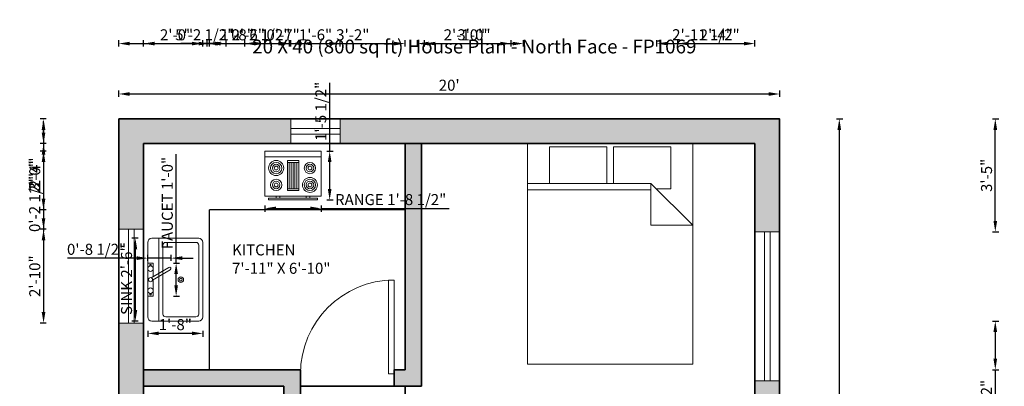
# Model space of a CAD drawing. Units: inches. Extents: x -35 to 322, y -513 to 50.
# Tile 3 of 3: x -35 to 322, y -83 to 50. Entities that reach past the tile are written whole.
import ezdxf

# ---------------------------------------------------------------- set-up
doc = ezdxf.new("R2010")
doc.units = ezdxf.units.IN
for name, color, linetype, lineweight in [('A-ANNO-DIMS', 2, 'Continuous', 18), ('A-ANNO-TEXT', 7, 'Continuous', 25), ('A-AREA-IDEN', 7, 'Continuous', 18), ('A-DOOR', 4, 'Continuous', 18), ('A-EQPM', 8, 'Continuous', 18), ('A-FLOR-CASE', 8, 'Continuous', 25), ('A-FLOR-FIXT', 9, 'Continuous', 18), ('A-FURN', 8, 'Continuous', 18), ('A-GLAZ', 6, 'Continuous', 18), ('A-WALL', 7, 'Continuous', 35), ('A-WALL-PATT', 251, 'Continuous', 13)]:
    doc.layers.add(name, color=color, linetype=linetype, lineweight=lineweight)
doc.styles.get("Standard").update_dxf_attribs({"font": 'arial.ttf'})
doc.dimstyles.new('ISO-25', dxfattribs={"dimtxt": 4, "dimasz": 4, "dimexe": 1.25, "dimexo": 0.625, "dimtad": 1, "dimlunit": 3, "dimtxsty": 'Standard', "dimcen": 2.5, "dimadec": 0, "dimazin": 0, "dimtfac": 1, "dimtmove": 0, "dimatfit": 3, "dimfxl": 1, "dimfxlon": 1, "dimarcsym": 0})

# ---------------------------------------------------------------- blocks, each defined once
blk = doc.blocks.new('*U4')
for p, q in [((0, 0), (0, -100)), ((750, 0), (750, -100))]:
    blk.add_line(p, q)
blk.add_lwpolyline([(0, 0), (0, 750), (43.75, 750), (43.75, 0)], close=True)
blk.add_arc((0, 0), 750, 0, 90)
blk = doc.blocks.new('Range-Oven - 30 in top')
for p, q in [((0, -3), (30, -3)), ((12, -6), (18, -6)), ((13, -20), (13, -6)), ((14, -6), (14, -20)), ((15, -20), (15, -6)), ((16, -6), (16, -20)), ((17, -20), (17, -6)), ((18, -20), (12, -20)), ((6, -24), (6, -25)), ((8, -25), (8, -24)), ((22, -25), (22, -24)), ((24, -24), (24, -25))]:
    blk.add_line(p, q)
for points in [[(0, -24), (0, 0), (30, 0), (30, -24)], [(12, -21), (12, -5), (18, -5), (18, -21)], [(2, -26), (2, -25), (28, -25), (28, -26)]]:
    blk.add_lwpolyline(points, close=True)
for centre, radius in [((6, -9), 4), ((6, -9), 3), ((6, -9), 2), ((6, -9), 1), ((24, -9), 3), ((24, -9), 2), ((24, -9), 1), ((6, -18), 3), ((24, -18), 4), ((24, -18), 3), ((6, -18), 2), ((6, -18), 1), ((24, -18), 2), ((24, -18), 1)]:
    blk.add_circle(centre, radius)
blk = doc.blocks.new('Sink-single - 30 in top')
blk.add_line((-15, -3.999996), (15, -3.999996))
for points in [[(-13.5, 0), (13.5, 0)], [(-15, -18.499996), (-15, -1.5)], [(15, -1.5), (15, -18.499996)], [(-13.5, -17.499996), (-13.5, -6.499996)], [(-12.5, -5.499996), (12.5, -5.499996)], [(13.5, -6.499996), (13.5, -17.499996)], [(13.5, -19.999996), (-13.5, -19.999996)], [(12.5, -18.499996), (-12.5, -18.499996)]]:
    blk.add_lwpolyline(points)
for radius in [1, 0.5]:
    blk.add_circle((0, -11.999996), radius)
for centre, radius, start, end in [((-13.5, -1.5), 1.5, 90, 180), ((13.5, -1.5), 1.5, 0, 90), ((-12.5, -6.499996), 1, 90, 180), ((12.5, -6.499996), 1, 0, 90), ((-12.5, -17.499996), 1, 180, 270), ((12.5, -17.499996), 1, 270, 0), ((-13.5, -18.499996), 1.5, 180, 270), ((13.5, -18.499996), 1.5, 270, 0)]:
    blk.add_arc(centre, radius, start, end)
blk = doc.blocks.new('Faucet - kit sink top')
for p, q in [((-5.5, -0.75), (-5.5, -1.25)), ((-4.94278, -0.75), (-5.5, -0.75)), ((-5.5, -1.25), (-4.94278, -1.25)), ((-0.14775, -1.7441), (3.56698, -8.1782)), ((4.43301, -7.6782), (0.71828, -1.2441)), ((4.94278, -0.75), (5.5, -0.75)), ((5.5, -1.25), (4.94278, -1.25)), ((5.5, -0.75), (5.5, -1.25))]:
    blk.add_line(p, q)
blk.add_lwpolyline([(-0.00587, -2), (-6, -2), (-6, 0), (6, 0), (6, -2), (1.15195, -2)])
for centre, radius in [((-4, -1), 1), ((4, -1), 1), ((0, -1), 0.75)]:
    blk.add_circle(centre, radius)
blk.add_arc((4, -7.9282), 0.5, 210, 30)
blk = doc.blocks.new('Bed - Queen')
for p, q in [((0, -80.00003), (0, 0)), ((0, 0), (59.99999, 0)), ((59.99999, 0), (59.99999, -80.00003)), ((7.99999, -1.2), (28.79998, -1.2)), ((7.99999, -14.4), (7.99999, -1.2)), ((28.79998, -1.2), (28.79998, -14.4)), ((31.19999, -1.2), (51.99999, -1.2)), ((31.19999, -14.4), (31.19999, -1.2)), ((51.99999, -1.2), (51.99999, -16.4)), ((0, -14.4), (44.8, -14.4)), ((44.8, -16.8), (0, -16.8)), ((59.99999, -29.6), (44.8, -14.4)), ((44.8, -14.4), (44.8, -29.6)), ((51.99999, -16.4), (46.79936, -16.4)), ((44.8, -29.6), (59.99999, -29.6)), ((59.99999, -80.00003), (0, -80.00003))]:
    blk.add_line(p, q)
blk = doc.blocks.new('*D12')
at = {"layer": 'A-ANNO-DIMS', "color": 0, "lineweight": -2, "transparency": 16777216}
for p, q in [((0.64, 22.01), (0.64, 24.26)), ((4.64, 23.01), (236.64, 23.01)), ((240.64, 22.01), (240.64, 24.26))]:
    blk.add_line(p, q, dxfattribs=at)
at = {"layer": 'A-ANNO-DIMS', "color": 0, "transparency": 16777216}
for points in [[(4.64, 23.67), (4.64, 22.34), (0.64, 23.01)], [(236.64, 23.67), (236.64, 22.34), (240.64, 23.01)]]:
    blk.add_solid(points, dxfattribs=at)
at = {"layer": 'Defpoints', "color": 0, "transparency": 16777216}
for p in [(240.64, 23.01), (0.64, 13.99), (240.64, 13.99)]:
    blk.add_point(p, dxfattribs=at)
at = {"layer": 'A-ANNO-DIMS', "color": 0, "transparency": 16777216, "insert": (120.64, 25.67), "char_height": 4, "attachment_point": 5}
blk.add_mtext("20'", dxfattribs=at)
blk = doc.blocks.new('*D13')
at = {"layer": 'A-ANNO-DIMS', "color": 0, "lineweight": -2, "transparency": 16777216}
for p, q in [((261.29, 13.99), (263.54, 13.99)), ((262.29, 9.99), (262.29, -462.01)), ((261.29, -466.01), (263.54, -466.01))]:
    blk.add_line(p, q, dxfattribs=at)
at = {"layer": 'A-ANNO-DIMS', "color": 0, "transparency": 16777216}
for points in [[(261.62, 9.99), (262.95, 9.99), (262.29, 13.99)], [(261.62, -462.01), (262.95, -462.01), (262.29, -466.01)]]:
    blk.add_solid(points, dxfattribs=at)
at = {"layer": 'Defpoints', "color": 0, "transparency": 16777216}
for p in [(239.43, 13.99), (240.64, -466.01), (262.29, -466.01)]:
    blk.add_point(p, dxfattribs=at)
at = {"layer": 'A-ANNO-DIMS', "color": 0, "transparency": 16777216, "insert": (259.62, -226.01), "char_height": 4, "attachment_point": 5, "rotation": 90}
blk.add_mtext("40'", dxfattribs=at)
blk = doc.blocks.new('WIN-54IN')
for p, q in [((3.5, 54), (3.5, 0)), ((5.5, 54), (5.5, 0))]:
    blk.add_line(p, q)
blk.add_lwpolyline([(0, 54), (9, 54), (9, 0), (0, 0)], close=True)
blk = doc.blocks.new('*D20')
at = {"layer": 'A-ANNO-DIMS', "color": 0, "lineweight": -2, "transparency": 16777216}
for p, q in [((53.72, -17.5), (53.72, -19.75)), ((74.17, -17.5), (74.17, -19.75)), ((57.72, -18.5), (70.17, -18.5)), ((74.17, -18.5), (120.59, -18.5))]:
    blk.add_line(p, q, dxfattribs=at)
at = {"layer": 'A-ANNO-DIMS', "color": 0, "transparency": 16777216}
for points in [[(57.72, -17.84), (57.72, -19.17), (53.72, -18.5)], [(70.17, -17.84), (70.17, -19.17), (74.17, -18.5)]]:
    blk.add_solid(points, dxfattribs=at)
at = {"layer": 'Defpoints', "color": 0, "transparency": 16777216}
for p in [(53.72, -15.44), (74.17, -15.44), (74.17, -18.5)]:
    blk.add_point(p, dxfattribs=at)
at = {"layer": 'A-ANNO-DIMS', "color": 0, "transparency": 16777216, "insert": (99.38, -15.81), "char_height": 4, "attachment_point": 5}
blk.add_mtext('RANGE 1\'-8 1/2"', dxfattribs=at)
blk = doc.blocks.new('*D21')
at = {"layer": 'A-ANNO-DIMS', "color": 0, "lineweight": -2, "transparency": 16777216}
for p, q in [((77.24, 2.28), (77.24, 27.11)), ((76.24, 2.28), (78.49, 2.28)), ((77.24, -11.44), (77.24, -1.72)), ((76.24, -15.44), (78.49, -15.44))]:
    blk.add_line(p, q, dxfattribs=at)
at = {"layer": 'A-ANNO-DIMS', "color": 0, "transparency": 16777216}
for points in [[(76.57, -1.72), (77.9, -1.72), (77.24, 2.28)], [(76.57, -11.44), (77.9, -11.44), (77.24, -15.44)]]:
    blk.add_solid(points, dxfattribs=at)
at = {"layer": 'Defpoints', "color": 0, "transparency": 16777216}
for p in [(74.17, 2.28), (77.24, 2.28), (74.17, -15.44)]:
    blk.add_point(p, dxfattribs=at)
at = {"layer": 'A-ANNO-DIMS', "color": 0, "transparency": 16777216, "insert": (74.54, 16.7), "char_height": 4, "attachment_point": 5, "rotation": 90}
blk.add_mtext('1\'-5 1/2"', dxfattribs=at)
blk = doc.blocks.new('*D22')
at = {"layer": 'A-ANNO-DIMS', "color": 0, "lineweight": -2, "transparency": 16777216}
for p, q in [((7.69, -29.34), (5.44, -29.34)), ((6.69, -55.34), (6.69, -33.34)), ((7.69, -59.34), (5.44, -59.34))]:
    blk.add_line(p, q, dxfattribs=at)
at = {"layer": 'A-ANNO-DIMS', "color": 0, "transparency": 16777216}
for points in [[(6.02, -33.34), (7.35, -33.34), (6.69, -29.34)], [(6.02, -55.34), (7.35, -55.34), (6.69, -59.34)]]:
    blk.add_solid(points, dxfattribs=at)
at = {"layer": 'Defpoints', "color": 0, "transparency": 16777216}
for p in [(6.69, -29.34), (11.19, -29.34), (11.19, -59.34)]:
    blk.add_point(p, dxfattribs=at)
at = {"layer": 'A-ANNO-DIMS', "color": 0, "transparency": 16777216, "insert": (3.99, -44.34), "char_height": 4, "attachment_point": 5, "rotation": 90}
blk.add_mtext('SINK 2\'-6"', dxfattribs=at)
blk = doc.blocks.new('*D23')
at = {"layer": 'A-ANNO-DIMS', "color": 0, "lineweight": -2, "transparency": 16777216}
for p, q in [((11.19, -62.84), (11.19, -65.09)), ((27.19, -63.84), (15.19, -63.84)), ((31.19, -62.84), (31.19, -65.09))]:
    blk.add_line(p, q, dxfattribs=at)
at = {"layer": 'A-ANNO-DIMS', "color": 0, "transparency": 16777216}
for points in [[(15.19, -63.17), (15.19, -64.51), (11.19, -63.84)], [(27.19, -63.17), (27.19, -64.51), (31.19, -63.84)]]:
    blk.add_solid(points, dxfattribs=at)
at = {"layer": 'Defpoints', "color": 0, "transparency": 16777216}
for p in [(11.19, -59.34), (31.19, -59.34), (11.19, -63.84)]:
    blk.add_point(p, dxfattribs=at)
at = {"layer": 'A-ANNO-DIMS', "color": 0, "transparency": 16777216, "insert": (21.19, -61.17), "char_height": 4, "attachment_point": 5}
blk.add_mtext('1\'-8"', dxfattribs=at)
blk = doc.blocks.new('*D24')
at = {"layer": 'A-ANNO-DIMS', "color": 0, "lineweight": -2, "transparency": 16777216}
for p, q in [((21.49, -38.34), (21.49, 1.22)), ((20.49, -38.34), (22.74, -38.34)), ((21.49, -46.34), (21.49, -42.34)), ((20.49, -50.34), (22.74, -50.34))]:
    blk.add_line(p, q, dxfattribs=at)
at = {"layer": 'A-ANNO-DIMS', "color": 0, "transparency": 16777216}
for points in [[(20.82, -42.34), (22.15, -42.34), (21.49, -38.34)], [(20.82, -46.34), (22.15, -46.34), (21.49, -50.34)]]:
    blk.add_solid(points, dxfattribs=at)
at = {"layer": 'Defpoints', "color": 0, "transparency": 16777216}
for p in [(19.69, -38.34), (21.49, -38.34), (19.69, -50.34)]:
    blk.add_point(p, dxfattribs=at)
at = {"layer": 'A-ANNO-DIMS', "color": 0, "transparency": 16777216, "insert": (18.79, -16.56), "char_height": 4, "attachment_point": 5, "rotation": 90}
blk.add_mtext('FAUCET 1\'-0"', dxfattribs=at)
blk = doc.blocks.new('*D25')
at = {"layer": 'A-ANNO-DIMS', "color": 0, "lineweight": -2, "transparency": 16777216}
for p, q in [((11.19, -37.54), (11.19, -35.29)), ((19.69, -37.54), (19.69, -35.29)), ((7.19, -36.54), (-18.02, -36.54)), ((19.69, -36.54), (11.19, -36.54)), ((23.69, -36.54), (27.69, -36.54))]:
    blk.add_line(p, q, dxfattribs=at)
at = {"layer": 'A-ANNO-DIMS', "color": 0, "transparency": 16777216}
for points in [[(7.19, -35.87), (7.19, -37.21), (11.19, -36.54)], [(23.69, -35.87), (23.69, -37.21), (19.69, -36.54)]]:
    blk.add_solid(points, dxfattribs=at)
at = {"layer": 'Defpoints', "color": 0, "transparency": 16777216}
for p in [(11.19, -36.54), (11.19, -38.34), (19.69, -38.34)]:
    blk.add_point(p, dxfattribs=at)
at = {"layer": 'A-ANNO-DIMS', "color": 0, "transparency": 16777216, "insert": (-7.41, -33.85), "char_height": 4, "attachment_point": 5}
blk.add_mtext('0\'-8 1/2"', dxfattribs=at)
blk = doc.blocks.new('*D26')
at = {"layer": 'A-ANNO-DIMS', "color": 0, "lineweight": -2, "transparency": 16777216}
for p, q in [((100.64, -509.7), (96.64, -509.7)), ((104.64, -508.7), (104.64, -510.95)), ((104.64, -509.7), (110.64, -509.7)), ((110.64, -508.7), (110.64, -510.95)), ((114.64, -509.7), (130.52, -509.7))]:
    blk.add_line(p, q, dxfattribs=at)
at = {"layer": 'A-ANNO-DIMS', "color": 0, "transparency": 16777216}
for points in [[(100.64, -509.04), (100.64, -510.37), (104.64, -509.7)], [(114.64, -509.04), (114.64, -510.37), (110.64, -509.7)]]:
    blk.add_solid(points, dxfattribs=at)
at = {"layer": 'Defpoints', "color": 0, "transparency": 16777216}
for p in [(104.64, -77.01), (110.64, -83.01), (110.64, -509.7)]:
    blk.add_point(p, dxfattribs=at)
at = {"layer": 'A-ANNO-DIMS', "color": 0, "transparency": 16777216, "insert": (124.58, -507.04), "char_height": 4, "attachment_point": 5}
blk.add_mtext('0\'-6"', dxfattribs=at)
blk = doc.blocks.new('*D29')
at = {"layer": 'A-ANNO-DIMS', "color": 0, "lineweight": -2, "transparency": 16777216}
for p, q in [((66.64, 40.29), (66.64, 42.54)), ((70.64, 41.29), (100.64, 41.29)), ((104.64, 40.29), (104.64, 42.54))]:
    blk.add_line(p, q, dxfattribs=at)
at = {"layer": 'A-ANNO-DIMS', "color": 0, "transparency": 16777216}
for points in [[(70.64, 41.95), (70.64, 40.62), (66.64, 41.29)], [(100.64, 41.95), (100.64, 40.62), (104.64, 41.29)]]:
    blk.add_solid(points, dxfattribs=at)
at = {"layer": 'Defpoints', "color": 0, "transparency": 16777216}
for p in [(104.64, 41.29), (66.64, -466.01), (104.64, -466.01)]:
    blk.add_point(p, dxfattribs=at)
at = {"layer": 'A-ANNO-DIMS', "color": 0, "transparency": 16777216, "insert": (85.64, 43.96), "char_height": 4, "attachment_point": 5}
blk.add_mtext('3\'-2"', dxfattribs=at)
blk = doc.blocks.new('*D31')
at = {"layer": 'A-ANNO-DIMS', "color": 0, "lineweight": -2, "transparency": 16777216}
for p, q in [((0.64, 40.29), (0.64, 42.54)), ((4.64, 41.29), (59.1, 41.29)), ((63.1, 40.29), (63.1, 42.54))]:
    blk.add_line(p, q, dxfattribs=at)
at = {"layer": 'A-ANNO-DIMS', "color": 0, "transparency": 16777216}
for points in [[(4.64, 41.95), (4.64, 40.62), (0.64, 41.29)], [(59.1, 41.95), (59.1, 40.62), (63.1, 41.29)]]:
    blk.add_solid(points, dxfattribs=at)
at = {"layer": 'Defpoints', "color": 0, "transparency": 16777216}
for p in [(63.1, 41.29), (0.64, 13.99), (63.1, 13.99)]:
    blk.add_point(p, dxfattribs=at)
at = {"layer": 'A-ANNO-DIMS', "color": 0, "transparency": 16777216, "insert": (31.87, 43.98), "char_height": 4, "attachment_point": 5}
blk.add_mtext('5\'-2 1/2"', dxfattribs=at)
blk = doc.blocks.new('*D32')
at = {"layer": 'A-ANNO-DIMS', "color": 0, "lineweight": -2, "transparency": 16777216}
for p, q in [((63.1, 40.29), (63.1, 42.54)), ((67.1, 41.29), (77.1, 41.29)), ((81.1, 40.29), (81.1, 42.54))]:
    blk.add_line(p, q, dxfattribs=at)
at = {"layer": 'A-ANNO-DIMS', "color": 0, "transparency": 16777216}
for points in [[(67.1, 41.95), (67.1, 40.62), (63.1, 41.29)], [(77.1, 41.95), (77.1, 40.62), (81.1, 41.29)]]:
    blk.add_solid(points, dxfattribs=at)
at = {"layer": 'Defpoints', "color": 0, "transparency": 16777216}
for p in [(81.1, 41.29), (63.1, 13.99), (81.1, 13.99)]:
    blk.add_point(p, dxfattribs=at)
at = {"layer": 'A-ANNO-DIMS', "color": 0, "transparency": 16777216, "insert": (72.1, 43.95), "char_height": 4, "attachment_point": 5}
blk.add_mtext('1\'-6"', dxfattribs=at)
blk = doc.blocks.new('*D33')
at = {"layer": 'A-ANNO-DIMS', "color": 0, "lineweight": -2, "transparency": 16777216}
for p, q in [((-25.66, 13.99), (-27.91, 13.99)), ((-26.66, 9.99), (-26.66, -22.08)), ((-25.66, -26.08), (-27.91, -26.08))]:
    blk.add_line(p, q, dxfattribs=at)
at = {"layer": 'A-ANNO-DIMS', "color": 0, "transparency": 16777216}
for points in [[(-27.33, 9.99), (-26, 9.99), (-26.66, 13.99)], [(-27.33, -22.08), (-26, -22.08), (-26.66, -26.08)]]:
    blk.add_solid(points, dxfattribs=at)
at = {"layer": 'Defpoints', "color": 0, "transparency": 16777216}
for p in [(0.64, 13.99), (-26.66, -26.08), (0.7, -26.08)]:
    blk.add_point(p, dxfattribs=at)
at = {"layer": 'A-ANNO-DIMS', "color": 0, "transparency": 16777216, "insert": (-29.33, -6.05), "char_height": 4, "attachment_point": 5, "rotation": 90}
blk.add_mtext('3\'-4"', dxfattribs=at)
blk = doc.blocks.new('*D34')
at = {"layer": 'A-ANNO-DIMS', "color": 0, "lineweight": -2, "transparency": 16777216}
for p, q in [((-25.66, -26.08), (-27.91, -26.08)), ((-26.66, -30.08), (-26.66, -56.08)), ((-25.66, -60.08), (-27.91, -60.08))]:
    blk.add_line(p, q, dxfattribs=at)
at = {"layer": 'A-ANNO-DIMS', "color": 0, "transparency": 16777216}
for points in [[(-27.33, -30.08), (-26, -30.08), (-26.66, -26.08)], [(-27.33, -56.08), (-26, -56.08), (-26.66, -60.08)]]:
    blk.add_solid(points, dxfattribs=at)
at = {"layer": 'Defpoints', "color": 0, "transparency": 16777216}
for p in [(0.7, -26.08), (-26.66, -60.08), (0.7, -60.08)]:
    blk.add_point(p, dxfattribs=at)
at = {"layer": 'A-ANNO-DIMS', "color": 0, "transparency": 16777216, "insert": (-29.33, -43.08), "char_height": 4, "attachment_point": 5, "rotation": 90}
blk.add_mtext('2\'-10"', dxfattribs=at)
blk = doc.blocks.new('*D38')
at = {"layer": 'A-ANNO-DIMS', "color": 0, "lineweight": -2, "transparency": 16777216}
for p, q in [((317.94, 13.99), (320.19, 13.99)), ((318.94, -23.02), (318.94, 9.99)), ((317.94, -27.02), (320.19, -27.02))]:
    blk.add_line(p, q, dxfattribs=at)
at = {"layer": 'A-ANNO-DIMS', "color": 0, "transparency": 16777216}
for points in [[(318.27, 9.99), (319.6, 9.99), (318.94, 13.99)], [(318.27, -23.02), (319.6, -23.02), (318.94, -27.02)]]:
    blk.add_solid(points, dxfattribs=at)
at = {"layer": 'Defpoints', "color": 0, "transparency": 16777216}
for p in [(240.64, 13.99), (318.94, 13.99), (240.64, -27.02)]:
    blk.add_point(p, dxfattribs=at)
at = {"layer": 'A-ANNO-DIMS', "color": 0, "transparency": 16777216, "insert": (316.27, -6.52), "char_height": 4, "attachment_point": 5, "rotation": 90}
blk.add_mtext('3\'-5"', dxfattribs=at)
blk = doc.blocks.new('*D42')
at = {"layer": 'A-ANNO-DIMS', "color": 0, "lineweight": -2, "transparency": 16777216}
for p, q in [((196.08, 40.29), (196.08, 42.54)), ((200.08, 41.29), (227.64, 41.29)), ((231.64, 40.29), (231.64, 42.54))]:
    blk.add_line(p, q, dxfattribs=at)
at = {"layer": 'A-ANNO-DIMS', "color": 0, "transparency": 16777216}
for points in [[(200.08, 41.95), (200.08, 40.62), (196.08, 41.29)], [(227.64, 41.95), (227.64, 40.62), (231.64, 41.29)]]:
    blk.add_solid(points, dxfattribs=at)
at = {"layer": 'Defpoints', "color": 0, "transparency": 16777216}
for p in [(231.64, 41.29), (196.08, -457.01), (231.64, -457.01)]:
    blk.add_point(p, dxfattribs=at)
at = {"layer": 'A-ANNO-DIMS', "color": 0, "transparency": 16777216, "insert": (213.86, 43.98), "char_height": 4, "attachment_point": 5}
blk.add_mtext('2\'-11 1/2"', dxfattribs=at)
blk = doc.blocks.new('*D44')
at = {"layer": 'A-ANNO-DIMS', "color": 0, "lineweight": -2, "transparency": 16777216}
for p, q in [((9.64, 40.29), (9.64, 42.54)), ((13.64, 41.29), (29.64, 41.29)), ((33.64, 40.29), (33.64, 42.54))]:
    blk.add_line(p, q, dxfattribs=at)
at = {"layer": 'A-ANNO-DIMS', "color": 0, "transparency": 16777216}
for points in [[(13.64, 41.95), (13.64, 40.62), (9.64, 41.29)], [(29.64, 41.95), (29.64, 40.62), (33.64, 41.29)]]:
    blk.add_solid(points, dxfattribs=at)
at = {"layer": 'Defpoints', "color": 0, "transparency": 16777216}
for p in [(33.64, 41.29), (9.64, -77.01), (33.64, -77.01)]:
    blk.add_point(p, dxfattribs=at)
at = {"layer": 'A-ANNO-DIMS', "color": 0, "transparency": 16777216, "insert": (21.64, 43.95), "char_height": 4, "attachment_point": 5}
blk.add_mtext('2\'-0"', dxfattribs=at)
blk = doc.blocks.new('*D45')
at = {"layer": 'A-ANNO-DIMS', "color": 0, "lineweight": -2, "transparency": 16777216}
for p, q in [((-25.66, 4.99), (-27.91, 4.99)), ((-26.66, 0.99), (-26.66, -15.01)), ((-25.66, -19.01), (-27.91, -19.01))]:
    blk.add_line(p, q, dxfattribs=at)
at = {"layer": 'A-ANNO-DIMS', "color": 0, "transparency": 16777216}
for points in [[(-27.33, 0.99), (-26, 0.99), (-26.66, 4.99)], [(-27.33, -15.01), (-26, -15.01), (-26.66, -19.01)]]:
    blk.add_solid(points, dxfattribs=at)
at = {"layer": 'Defpoints', "color": 0, "transparency": 16777216}
for p in [(104.64, 4.99), (-26.66, -19.01), (104.64, -19.01)]:
    blk.add_point(p, dxfattribs=at)
at = {"layer": 'A-ANNO-DIMS', "color": 0, "transparency": 16777216, "insert": (-29.33, -7.01), "char_height": 4, "attachment_point": 5, "rotation": 90}
blk.add_mtext('2\'-0"', dxfattribs=at)
blk = doc.blocks.new('*D46')
at = {"layer": 'A-ANNO-DIMS', "color": 0, "lineweight": -2, "transparency": 16777216}
for p, q in [((32.73, 40.29), (32.73, 42.54)), ((36.73, 41.29), (58.65, 41.29)), ((62.65, 40.29), (62.65, 42.54))]:
    blk.add_line(p, q, dxfattribs=at)
at = {"layer": 'A-ANNO-DIMS', "color": 0, "transparency": 16777216}
for points in [[(36.73, 41.95), (36.73, 40.62), (32.73, 41.29)], [(58.65, 41.95), (58.65, 40.62), (62.65, 41.29)]]:
    blk.add_solid(points, dxfattribs=at)
at = {"layer": 'Defpoints', "color": 0, "transparency": 16777216}
for p in [(62.65, 41.29), (32.73, -162.01), (62.65, -162.01)]:
    blk.add_point(p, dxfattribs=at)
at = {"layer": 'A-ANNO-DIMS', "color": 0, "transparency": 16777216, "insert": (47.69, 43.95), "char_height": 4, "attachment_point": 5}
blk.add_mtext('2\'-6"', dxfattribs=at)
blk = doc.blocks.new('*D47')
at = {"layer": 'A-ANNO-DIMS', "color": 0, "lineweight": -2, "transparency": 16777216}
for p, q in [((109.17, 40.29), (109.17, 42.54)), ((113.17, 41.29), (139.16, 41.29)), ((143.16, 40.29), (143.16, 42.54))]:
    blk.add_line(p, q, dxfattribs=at)
at = {"layer": 'A-ANNO-DIMS', "color": 0, "transparency": 16777216}
for points in [[(113.17, 41.95), (113.17, 40.62), (109.17, 41.29)], [(139.16, 41.95), (139.16, 40.62), (143.16, 41.29)]]:
    blk.add_solid(points, dxfattribs=at)
at = {"layer": 'Defpoints', "color": 0, "transparency": 16777216}
for p in [(143.16, 41.29), (109.17, -117.01), (143.16, -117.01)]:
    blk.add_point(p, dxfattribs=at)
at = {"layer": 'A-ANNO-DIMS', "color": 0, "transparency": 16777216, "insert": (126.17, 43.95), "char_height": 4, "attachment_point": 5}
blk.add_mtext('2\'-10"', dxfattribs=at)
blk = doc.blocks.new('*D50')
at = {"layer": 'A-ANNO-DIMS', "color": 0, "lineweight": -2, "transparency": 16777216}
for p, q in [((111.64, 40.29), (111.64, 42.54)), ((115.64, 41.29), (143.64, 41.29)), ((147.64, 40.29), (147.64, 42.54))]:
    blk.add_line(p, q, dxfattribs=at)
at = {"layer": 'A-ANNO-DIMS', "color": 0, "transparency": 16777216}
for points in [[(115.64, 41.95), (115.64, 40.62), (111.64, 41.29)], [(143.64, 41.95), (143.64, 40.62), (147.64, 41.29)]]:
    blk.add_solid(points, dxfattribs=at)
at = {"layer": 'Defpoints', "color": 0, "transparency": 16777216}
for p in [(147.64, 41.29), (111.64, -320.01), (147.64, -320.01)]:
    blk.add_point(p, dxfattribs=at)
at = {"layer": 'A-ANNO-DIMS', "color": 0, "transparency": 16777216, "insert": (129.64, 43.96), "char_height": 4, "attachment_point": 5}
blk.add_mtext('3\'-0"', dxfattribs=at)
blk = doc.blocks.new('*D51')
at = {"layer": 'A-ANNO-DIMS', "color": 0, "lineweight": -2, "transparency": 16777216}
for p, q in [((203.64, 40.29), (203.64, 42.54)), ((207.64, 41.29), (227.64, 41.29)), ((231.64, 40.29), (231.64, 42.54))]:
    blk.add_line(p, q, dxfattribs=at)
at = {"layer": 'A-ANNO-DIMS', "color": 0, "transparency": 16777216}
for points in [[(207.64, 41.95), (207.64, 40.62), (203.64, 41.29)], [(227.64, 41.95), (227.64, 40.62), (231.64, 41.29)]]:
    blk.add_solid(points, dxfattribs=at)
at = {"layer": 'Defpoints', "color": 0, "transparency": 16777216}
for p in [(231.64, 41.29), (231.64, -295.18), (203.64, -305.68)]:
    blk.add_point(p, dxfattribs=at)
at = {"layer": 'A-ANNO-DIMS', "color": 0, "transparency": 16777216, "insert": (217.64, 43.92), "char_height": 4, "attachment_point": 5}
blk.add_mtext('2\'-4"', dxfattribs=at)
blk = doc.blocks.new('*D54')
at = {"layer": 'A-ANNO-DIMS', "color": 0, "lineweight": -2, "transparency": 16777216}
for p, q in [((209.06, -508.7), (209.06, -510.95)), ((213.06, -509.7), (227.64, -509.7)), ((231.64, -508.7), (231.64, -510.95)), ((231.64, -509.7), (259.57, -509.7))]:
    blk.add_line(p, q, dxfattribs=at)
at = {"layer": 'A-ANNO-DIMS', "color": 0, "transparency": 16777216}
for points in [[(213.06, -509.04), (213.06, -510.37), (209.06, -509.7)], [(227.64, -509.04), (227.64, -510.37), (231.64, -509.7)]]:
    blk.add_solid(points, dxfattribs=at)
at = {"layer": 'Defpoints', "color": 0, "transparency": 16777216}
for p in [(209.06, 4.99), (231.64, 4.99), (231.64, -509.7)]:
    blk.add_point(p, dxfattribs=at)
at = {"layer": 'A-ANNO-DIMS', "color": 0, "transparency": 16777216, "insert": (247.6, -507.01), "char_height": 4, "attachment_point": 5}
blk.add_mtext('1\'-10 1/2"', dxfattribs=at)
blk = doc.blocks.new('*D57')
at = {"layer": 'A-ANNO-DIMS', "color": 0, "lineweight": -2, "transparency": 16777216}
for p, q in [((33.64, 40.29), (33.64, 42.54)), ((37.64, 41.29), (49.72, 41.29)), ((53.72, 40.29), (53.72, 42.54))]:
    blk.add_line(p, q, dxfattribs=at)
at = {"layer": 'A-ANNO-DIMS', "color": 0, "transparency": 16777216}
for points in [[(37.64, 41.95), (37.64, 40.62), (33.64, 41.29)], [(49.72, 41.95), (49.72, 40.62), (53.72, 41.29)]]:
    blk.add_solid(points, dxfattribs=at)
at = {"layer": 'Defpoints', "color": 0, "transparency": 16777216}
for p in [(53.72, 41.29), (53.72, -14.07), (33.64, -19.01)]:
    blk.add_point(p, dxfattribs=at)
at = {"layer": 'A-ANNO-DIMS', "color": 0, "transparency": 16777216, "insert": (43.68, 43.95), "char_height": 4, "attachment_point": 5}
blk.add_mtext('1\'-8"', dxfattribs=at)
blk = doc.blocks.new('*D58')
at = {"layer": 'A-ANNO-DIMS', "color": 0, "lineweight": -2, "transparency": 16777216}
for p, q in [((-26.66, 8.99), (-26.66, 12.99)), ((-25.66, 4.99), (-27.91, 4.99)), ((-26.66, 4.99), (-26.66, 2.28)), ((-25.66, 2.28), (-27.91, 2.28)), ((-26.66, -1.72), (-26.66, -26.92))]:
    blk.add_line(p, q, dxfattribs=at)
at = {"layer": 'A-ANNO-DIMS', "color": 0, "transparency": 16777216}
for points in [[(-27.33, 8.99), (-26, 8.99), (-26.66, 4.99)], [(-27.33, -1.72), (-26, -1.72), (-26.66, 2.28)]]:
    blk.add_solid(points, dxfattribs=at)
at = {"layer": 'Defpoints', "color": 0, "transparency": 16777216}
for p in [(63.1, 4.99), (-26.66, 2.28), (53.72, 2.28)]:
    blk.add_point(p, dxfattribs=at)
at = {"layer": 'A-ANNO-DIMS', "color": 0, "transparency": 16777216, "insert": (-29.36, -16.32), "char_height": 4, "attachment_point": 5, "rotation": 90}
blk.add_mtext('0\'-2 1/2"', dxfattribs=at)
blk = doc.blocks.new('*D59')
at = {"layer": 'A-ANNO-DIMS', "color": 0, "lineweight": -2, "transparency": 16777216}
for p, q in [((317.94, -59.34), (320.19, -59.34)), ((318.94, -63.34), (318.94, -73.01)), ((317.94, -77.01), (320.19, -77.01)), ((318.94, -77.01), (318.94, -101.84))]:
    blk.add_line(p, q, dxfattribs=at)
at = {"layer": 'A-ANNO-DIMS', "color": 0, "transparency": 16777216}
for points in [[(318.27, -63.34), (319.6, -63.34), (318.94, -59.34)], [(318.27, -73.01), (319.6, -73.01), (318.94, -77.01)]]:
    blk.add_solid(points, dxfattribs=at)
at = {"layer": 'Defpoints', "color": 0, "transparency": 16777216}
for p in [(29.69, -59.34), (33.64, -77.01), (318.94, -77.01)]:
    blk.add_point(p, dxfattribs=at)
at = {"layer": 'A-ANNO-DIMS', "color": 0, "transparency": 16777216, "insert": (316.24, -91.43), "char_height": 4, "attachment_point": 5, "rotation": 90}
blk.add_mtext('1\'-5 1/2"', dxfattribs=at)
blk = doc.blocks.new('*D60')
at = {"layer": 'A-ANNO-DIMS', "color": 0, "lineweight": -2, "transparency": 16777216}
for p, q in [((27.19, 41.29), (23.19, 41.29)), ((31.19, 40.29), (31.19, 42.54)), ((31.19, 41.29), (33.64, 41.29)), ((33.64, 40.29), (33.64, 42.54)), ((37.64, 41.29), (62.84, 41.29))]:
    blk.add_line(p, q, dxfattribs=at)
at = {"layer": 'A-ANNO-DIMS', "color": 0, "transparency": 16777216}
for points in [[(27.19, 41.95), (27.19, 40.62), (31.19, 41.29)], [(37.64, 41.95), (37.64, 40.62), (33.64, 41.29)]]:
    blk.add_solid(points, dxfattribs=at)
at = {"layer": 'Defpoints', "color": 0, "transparency": 16777216}
for p in [(33.64, 41.29), (31.19, -57.84), (33.64, -77.01)]:
    blk.add_point(p, dxfattribs=at)
at = {"layer": 'A-ANNO-DIMS', "color": 0, "transparency": 16777216, "insert": (52.24, 43.98), "char_height": 4, "attachment_point": 5}
blk.add_mtext('0\'-2 1/2"', dxfattribs=at)
blk = doc.blocks.new('*D61')
at = {"layer": 'A-ANNO-DIMS', "color": 0, "lineweight": -2, "transparency": 16777216}
for p, q in [((35.64, 41.29), (31.64, 41.29)), ((39.64, 40.29), (39.64, 42.54)), ((39.64, 41.29), (46.39, 41.29)), ((46.39, 40.29), (46.39, 42.54)), ((50.39, 41.29), (66.27, 41.29))]:
    blk.add_line(p, q, dxfattribs=at)
at = {"layer": 'A-ANNO-DIMS', "color": 0, "transparency": 16777216}
for points in [[(35.64, 41.95), (35.64, 40.62), (39.64, 41.29)], [(50.39, 41.95), (50.39, 40.62), (46.39, 41.29)]]:
    blk.add_solid(points, dxfattribs=at)
at = {"layer": 'Defpoints', "color": 0, "transparency": 16777216}
for p in [(46.39, 41.29), (39.64, -326.01), (46.39, -326.01)]:
    blk.add_point(p, dxfattribs=at)
at = {"layer": 'A-ANNO-DIMS', "color": 0, "transparency": 16777216, "insert": (60.33, 43.95), "char_height": 4, "attachment_point": 5}
blk.add_mtext('0\'-7"', dxfattribs=at)

msp = doc.modelspace()

# ---------------------------------------------------------------- hatches: boundary and pattern name
at = {"layer": 'A-WALL-PATT'}
h = msp.add_hatch(color=256, dxfattribs=at)
h.dxf.hatch_style = 1
h.paths.add_polyline_path([(63.099, 13.987), (0.637, 13.987), (0.637, -26.079), (9.637, -26.079), (9.637, 4.987), (63.099, 4.987)])
h.paths.add_polyline_path([(9.637, -107.554), (0.637, -107.554), (0.637, -205.04), (9.637, -205.04)])
h.paths.add_polyline_path([(9.637, -60.079), (0.637, -60.079), (0.637, -89.554), (9.637, -89.554)])
h.paths.add_polyline_path([(9.637, -259.04), (0.637, -259.04), (0.637, -466.013), (66.468, -466.013), (66.468, -460.924, -0.0235925), (66.637, -457.328), (66.637, -457.013), (9.637, -457.013), (9.637, -326.013)])
h.paths.add_polyline_path([(142.082, -457.013), (104.637, -457.013), (104.637, -460.924), (104.637, -466.013), (142.082, -466.013)])
h.paths.add_polyline_path([(240.637, -224.716), (231.637, -224.716), (231.637, -274.623), (240.637, -274.623)])
h.paths.add_polyline_path([(69.474, -113.132), (98.939, -113.132), (98.939, -98.154), (69.474, -98.154)], flags=9)
h.paths.add_polyline_path([(38.843, -240.589), (73.258, -240.589), (73.258, -225.663), (38.843, -225.663)], flags=9)
h.paths.add_polyline_path([(51.03, -393.995), (85.248, -393.995), (85.248, -379.069), (51.03, -379.069)], flags=9)
h.paths.add_polyline_path([(75.428, -462.589), (96.367, -462.589), (96.367, -454.346), (75.428, -454.346)], flags=9)
h.paths.add_polyline_path([(154.313, -353.536), (191.907, -353.536), (191.907, -338.61), (154.313, -338.61)], flags=9)
h.paths.add_polyline_path([(177.411, -284.106), (208.497, -284.106), (208.497, -269.18), (177.411, -269.18)], flags=9)
h.paths.add_polyline_path([(152.205, -160.654), (189.798, -160.654), (189.798, -145.728), (152.205, -145.728)], flags=9)
h.paths.add_polyline_path([(150.351, -98.334), (187.945, -98.334), (187.945, -83.408), (150.351, -83.408)], flags=9)
h.paths.add_polyline_path([(15.293, -117.178), (49.667, -117.178), (49.667, -102.252), (15.293, -102.252)], flags=9)
h.paths.add_polyline_path([(40.377, -44.483), (77.823, -44.483), (77.823, -29.557), (40.377, -29.557)], flags=9)
h.paths.add_polyline_path([(31.67, -336.447), (44.796, -336.447), (44.796, -328.204), (31.67, -328.204)], flags=25)
h = msp.add_hatch(color=256, dxfattribs=at)
h.dxf.hatch_style = 1
h.paths.add_polyline_path([(110.637, -167.013), (104.637, -167.013), (104.637, -265.013), (151.637, -265.013), (151.637, -286.013), (157.637, -286.013), (157.637, -265.013), (231.637, -265.013), (231.637, -259.013), (110.637, -259.013)])
h.paths.add_polyline_path([(240.637, 13.987), (81.099, 13.987), (81.099, 4.987), (104.637, 4.987), (110.637, 4.987), (231.637, 4.987), (231.637, -27.021), (240.637, -27.021)])
h = msp.add_hatch(color=256, dxfattribs=at)
h.dxf.hatch_style = 1
h.paths.add_polyline_path([(110.637, 4.987), (104.637, 4.987), (104.637, -77.013), (100.637, -77.013), (100.637, -78.48), (100.637, -83.013), (104.637, -83.013), (110.637, -83.013)])
h.paths.add_polyline_path([(231.637, -121.013), (110.637, -121.013), (110.637, -117.013), (109.17, -117.013), (104.637, -117.013), (104.637, -131.013), (110.637, -131.013), (110.637, -127.013), (231.637, -127.013)])
h.paths.add_polyline_path([(15.293, -117.178), (49.667, -117.178), (49.667, -102.252), (15.293, -102.252)], flags=9)
h.paths.add_polyline_path([(69.474, -113.132), (98.939, -113.132), (98.939, -98.154), (69.474, -98.154)], flags=9)
h.paths.add_polyline_path([(38.843, -240.589), (73.258, -240.589), (73.258, -225.663), (38.843, -225.663)], flags=9)
h.paths.add_polyline_path([(51.03, -393.995), (85.248, -393.995), (85.248, -379.069), (51.03, -379.069)], flags=9)
h.paths.add_polyline_path([(75.428, -462.589), (96.367, -462.589), (96.367, -454.346), (75.428, -454.346)], flags=9)
h.paths.add_polyline_path([(154.313, -353.536), (191.907, -353.536), (191.907, -338.61), (154.313, -338.61)], flags=9)
h.paths.add_polyline_path([(177.411, -284.106), (208.497, -284.106), (208.497, -269.18), (177.411, -269.18)], flags=9)
h.paths.add_polyline_path([(152.205, -160.654), (189.798, -160.654), (189.798, -145.728), (152.205, -145.728)], flags=9)
h.paths.add_polyline_path([(150.351, -98.334), (187.945, -98.334), (187.945, -83.408), (150.351, -83.408)], flags=9)
h.paths.add_polyline_path([(40.377, -44.483), (77.823, -44.483), (77.823, -29.557), (40.377, -29.557)], flags=9)
h = msp.add_hatch(color=256, dxfattribs=at)
h.dxf.hatch_style = 1
h.paths.add_polyline_path([(110.637, -326.013), (111.637, -326.013), (111.637, -324.8), (111.637, -320.013), (104.637, -320.013), (104.637, -457.013), (110.637, -457.013)])
h.paths.add_polyline_path([(231.637, -320.013), (157.637, -320.013), (157.637, -316.013), (153.631, -316.013), (151.637, -316.029), (151.637, -320.013), (147.637, -320.013), (147.637, -326.013), (151.637, -326.013), (157.637, -326.013), (231.637, -326.013)])
h.paths.add_polyline_path([(240.637, -292.623), (231.637, -292.623), (231.637, -457.013), (196.082, -457.013), (196.082, -466.013), (240.637, -466.013)])
h.paths.add_polyline_path([(15.293, -117.178), (49.667, -117.178), (49.667, -102.252), (15.293, -102.252)], flags=9)
h.paths.add_polyline_path([(69.474, -113.132), (98.939, -113.132), (98.939, -98.154), (69.474, -98.154)], flags=9)
h.paths.add_polyline_path([(38.843, -240.589), (73.258, -240.589), (73.258, -225.663), (38.843, -225.663)], flags=9)
h.paths.add_polyline_path([(51.03, -393.995), (85.248, -393.995), (85.248, -379.069), (51.03, -379.069)], flags=9)
h.paths.add_polyline_path([(75.428, -462.589), (96.367, -462.589), (96.367, -454.346), (75.428, -454.346)], flags=9)
h.paths.add_polyline_path([(154.313, -353.536), (191.907, -353.536), (191.907, -338.61), (154.313, -338.61)], flags=9)
h.paths.add_polyline_path([(152.205, -160.654), (189.798, -160.654), (189.798, -145.728), (152.205, -145.728)], flags=9)
h.paths.add_polyline_path([(150.351, -98.334), (187.945, -98.334), (187.945, -83.408), (150.351, -83.408)], flags=9)
h.paths.add_polyline_path([(40.377, -44.483), (77.823, -44.483), (77.823, -29.557), (40.377, -29.557)], flags=9)
h = msp.add_hatch(color=256, dxfattribs=at)
h.dxf.hatch_style = 1
h.paths.add_polyline_path([(66.637, -77.013), (9.637, -77.013), (9.637, -83.013), (60.637, -83.013), (60.637, -132.013), (66.637, -132.013), (66.637, -83.013), (66.636, -78.48)])
h.paths.add_polyline_path([(66.637, -162.013), (62.648, -162.013), (60.637, -162.013), (60.637, -166.013), (9.637, -166.013), (9.637, -172.013), (60.637, -172.013), (66.637, -172.013)])
h = msp.add_hatch(color=256, dxfattribs=at)
h.dxf.hatch_style = 1
h.paths.add_polyline_path([(240.637, -81.021), (231.637, -81.021), (231.637, -170.716), (240.637, -170.716)])

# ---------------------------------------------------------------- linework, layer by layer
at = {"layer": 'A-FLOR-CASE'}
for p in [(104.637, -19.013), (33.637, -77.013)]:
    msp.add_line(p, (33.637, -19.013), dxfattribs=at)
at = {"layer": 'A-GLAZ'}
for p, q in [((81.099, 10.487), (63.099, 10.487)), ((81.099, 8.487), (63.099, 8.487)), ((4.203, -26.079), (4.203, -60.079)), ((6.203, -26.079), (6.203, -60.079))]:
    msp.add_line(p, q, dxfattribs=at)
for points in [[(81.099, 13.987), (81.099, 4.987), (63.099, 4.987), (63.099, 13.987)], [(0.703, -26.079), (9.703, -26.079), (9.703, -60.079), (0.703, -60.079)]]:
    msp.add_lwpolyline(points, close=True, dxfattribs=at)
at = {"layer": 'A-WALL'}
for p, q in [((9.637, 4.987), (104.637, 4.987)), ((9.637, -326.013), (9.637, 4.987)), ((104.637, 4.987), (110.637, 4.987)), ((104.637, -77.013), (104.637, 4.987)), ((110.637, 4.987), (231.637, 4.987)), ((110.637, -83.013), (110.637, 4.987)), ((231.637, 4.987), (231.637, -457.013)), ((9.637, -77.013), (66.637, -77.013)), ((66.637, -83.013), (66.637, -77.013)), ((100.637, -77.013), (100.637, -83.013)), ((100.637, -77.013), (104.637, -77.013)), ((9.637, -83.013), (60.637, -83.013)), ((60.637, -83.013), (60.637, -132.013)), ((66.637, -83.013), (66.637, -172.013)), ((66.637, -83.013), (104.637, -83.013)), ((104.637, -83.013), (110.637, -83.013)), ((104.637, -265.013), (104.637, -83.013))]:
    msp.add_line(p, q, dxfattribs=at)
msp.add_lwpolyline([(0.637, 13.987), (240.637, 13.987), (240.637, -466.013), (0.637, -466.013)], close=True, dxfattribs=at)

# ---------------------------------------------------------------- block references
at = {"layer": 'A-DOOR', "xscale": -0.0453355142688786, "yscale": 0.0453355142688786, "zscale": 0.0453355142688786}
msp.add_blockref('*U4', (100.637, -78.48), dxfattribs=at)
at = {"layer": 'A-EQPM', "xscale": 0.681589820472302, "yscale": 0.681589820472302, "zscale": 0.681589820472302}
msp.add_blockref('Range-Oven - 30 in top', (53.722, 2.284), dxfattribs=at)
at = {"layer": 'A-FLOR-FIXT', "rotation": 90}
for name in ['Sink-single - 30 in top', 'Faucet - kit sink top']:
    msp.add_blockref(name, (11.187, -44.339), dxfattribs=at)
at = {"layer": 'A-FURN'}
msp.add_blockref('Bed - Queen', (149.063, 4.987), dxfattribs=at)
at = {"layer": 'A-GLAZ'}
msp.add_blockref('WIN-54IN', (231.637, -81.021), dxfattribs=at)

# ---------------------------------------------------------------- texts
at = {"layer": 'A-ANNO-TEXT', "insert": (49.131, 42.72), "char_height": 5, "attachment_point": 1}
msp.add_mtext_dynamic_manual_height_columns('20 X 40 (800 sq ft) House Plan - North Face - FP1069', width=226.60033, gutter_width=12.5, heights=[0], dxfattribs=at)
at = {"layer": 'A-AREA-IDEN', "insert": (41.786, -31.547), "char_height": 4, "attachment_point": 1}
msp.add_mtext_dynamic_manual_height_columns('KITCHEN\\P7\'-11" X 6\'-10"', width=44.68223, gutter_width=12.5, heights=[0], dxfattribs=at)

# ---------------------------------------------------------------- dimensions: what is measured, and where the dimension line sits
at = {"layer": 'A-ANNO-DIMS'}
for base, p1, p2, override, picture, middle in [((63.099, 41.287), (0.637, 13.987), (63.099, 13.987), {"dimdec": 1, "dimlfac": 1, "dimrnd": 0, "dimzin": 1, "dimdsep": 46, "dimlunit": 4, "dimfrac": 2}, '*D31', (31.868, 43.98)), ((33.637, 41.287), (9.637, -77.013), (33.637, -77.013), {"dimdec": 1, "dimlfac": 1, "dimrnd": 0, "dimzin": 1, "dimdsep": 46, "dimlunit": 4, "dimfrac": 2}, '*D44', (21.637, 43.954)), ((33.63744, 41.28691), (31.18743, -57.83919), (33.63744, -77.01309), {"dimdec": 1, "dimlfac": 1, "dimrnd": 0, "dimzin": 1, "dimdsep": 46, "dimlunit": 4, "dimfrac": 2}, '*D60', (52.23925, 43.98012)), ((46.387441, 41.286907), (39.637441, -326.013093), (46.387441, -326.013093), {"dimdec": 1, "dimlfac": 1, "dimrnd": 0, "dimzin": 1, "dimdsep": 46, "dimlunit": 4, "dimfrac": 2}, '*D61', (60.328948503, 43.954198951)), ((62.648, 41.287), (32.726, -162.013), (62.648, -162.013), {"dimdec": 1, "dimlfac": 1, "dimrnd": 0, "dimzin": 1, "dimdsep": 46, "dimlunit": 4, "dimfrac": 2}, '*D46', (47.687, 43.954)), ((53.722, 41.287), (33.637, -19.013), (53.722, -14.074), {"dimdec": 1, "dimlfac": 1, "dimrnd": 0, "dimzin": 1, "dimdsep": 46, "dimlunit": 4, "dimfrac": 2}, '*D57', (43.68, 43.954)), ((81.099, 41.287), (63.099, 13.987), (81.099, 13.987), {"dimdec": 1, "dimlfac": 1, "dimrnd": 0, "dimzin": 1, "dimdsep": 46, "dimlunit": 4, "dimfrac": 2}, '*D32', (72.099, 43.954)), ((104.637, 41.287), (66.637, -466.013), (104.637, -466.013), {"dimdec": 1, "dimlfac": 1, "dimrnd": 0, "dimzin": 1, "dimdsep": 46, "dimlunit": 4, "dimfrac": 2}, '*D29', (85.637, 43.956)), ((143.163, 41.287), (109.17, -117.013), (143.163, -117.013), {"dimdec": 1, "dimlfac": 1, "dimrnd": 0, "dimzin": 1, "dimdsep": 46, "dimlunit": 4, "dimfrac": 2}, '*D47', (126.167, 43.954)), ((147.637, 41.287), (111.637, -320.013), (147.637, -320.013), {"dimdec": 1, "dimlfac": 1, "dimrnd": 0, "dimzin": 1, "dimdsep": 46, "dimlunit": 4, "dimfrac": 2}, '*D50', (129.637, 43.956)), ((231.637, 41.287), (196.082, -457.013), (231.637, -457.013), {"dimdec": 1, "dimlfac": 1, "dimrnd": 0, "dimzin": 1, "dimdsep": 46, "dimlunit": 4, "dimfrac": 2}, '*D42', (213.86, 43.98)), ((231.637, 41.287), (203.637, -305.675), (231.637, -295.175), {"dimdec": 1, "dimlfac": 1, "dimrnd": 0, "dimzin": 1, "dimdsep": 46, "dimlunit": 4, "dimfrac": 2}, '*D51', (217.637, 43.92)), ((240.637, 23.005), (0.637, 13.987), (240.637, 13.987), {"dimclrd": 0, "dimclre": 0, "dimclrt": 0}, '*D12', (120.637, 25.672)), ((231.637, -509.704), (209.063, 4.987), (231.637, 4.987), {"dimdec": 1, "dimlfac": 1, "dimrnd": 0, "dimzin": 1, "dimdsep": 46, "dimlunit": 4, "dimfrac": 2}, '*D54', (247.605, -507.011)), ((110.637, -509.704), (104.637, -77.013), (110.637, -83.013), {"dimdec": 1, "dimlfac": 1, "dimrnd": 0, "dimzin": 1, "dimdsep": 46, "dimlunit": 4, "dimfrac": 2}, '*D26', (124.579, -507.037))]:
    dim = msp.add_linear_dim(base=base, p1=p1, p2=p2, dimstyle='ISO-25', override=override, dxfattribs=at)
    dim.commit()
    dim.dimension.update_dxf_attribs({"geometry": picture, "text_midpoint": middle})
for base, p1, p2, angle, override, picture, middle in [((77.236, 2.284), (74.169, -15.437), (74.169, 2.284), 90, {"dimdec": 1, "dimlfac": 1, "dimrnd": 0, "dimzin": 1, "dimdsep": 46, "dimlunit": 4, "dimfrac": 2}, '*D21', (74.543, 16.698)), ((-26.663, 2.284), (63.099, 4.987), (53.722, 2.284), 90, {"dimdec": 1, "dimlfac": 1, "dimrnd": 0, "dimzin": 1, "dimdsep": 46, "dimlunit": 4, "dimfrac": 2}, '*D58', (-29.356, -16.318)), ((-26.663, -26.079), (0.637, 13.987), (0.703, -26.079), 90, {"dimdec": 1, "dimlfac": 1, "dimrnd": 0, "dimzin": 1, "dimdsep": 46, "dimlunit": 4, "dimfrac": 2}, '*D33', (-29.331, -6.046)), ((262.288, -466.013), (239.425, 13.987), (240.637, -466.013), 90, {"dimclrd": 0, "dimclre": 0, "dimclrt": 0}, '*D13', (259.621, -226.013)), ((318.937, 13.987), (240.637, -27.021), (240.637, 13.987), 90, {"dimdec": 1, "dimlfac": 1, "dimrnd": 0, "dimzin": 1, "dimdsep": 46, "dimlunit": 4, "dimfrac": 2}, '*D38', (316.269, -6.517)), ((-26.663, -19.013), (104.637, 4.987), (104.637, -19.013), 90, {"dimdec": 1, "dimlfac": 1, "dimrnd": 0, "dimzin": 1, "dimdsep": 46, "dimlunit": 4, "dimfrac": 2}, '*D45', (-29.33, -7.013)), ((-26.663, -60.079), (0.703, -26.079), (0.703, -60.079), 90, {"dimdec": 1, "dimlfac": 1, "dimrnd": 0, "dimzin": 1, "dimdsep": 46, "dimlunit": 4, "dimfrac": 2}, '*D34', (-29.33, -43.079)), ((11.187, -36.539), (19.687, -38.339), (11.187, -38.339), 180, {"dimdec": 1, "dimlfac": 1, "dimrnd": 0, "dimzin": 1, "dimdsep": 46, "dimlunit": 4, "dimfrac": 2}, '*D25', (-7.414, -33.846)), ((11.187, -63.839), (31.187, -59.339), (11.187, -59.339), 180, {"dimdec": 1, "dimlfac": 1, "dimrnd": 0, "dimzin": 1, "dimdsep": 46, "dimlunit": 4, "dimfrac": 2}, '*D23', (21.187, -61.172)), ((318.937, -77.013), (29.687, -59.339), (33.637, -77.013), 90, {"dimdec": 1, "dimlfac": 1, "dimrnd": 0, "dimzin": 1, "dimdsep": 46, "dimlunit": 4, "dimfrac": 2}, '*D59', (316.244, -91.427))]:
    dim = msp.add_linear_dim(base=base, p1=p1, p2=p2, angle=angle, dimstyle='ISO-25', override=override, dxfattribs=at)
    dim.commit()
    dim.dimension.update_dxf_attribs({"geometry": picture, "text_midpoint": middle})
for base, p1, p2, text, picture, middle in [((21.487, -38.339), (19.687, -50.339), (19.687, -38.339), 'FAUCET <>', '*D24', (18.794, -16.559)), ((6.687, -29.339), (11.187, -59.339), (11.187, -29.339), 'SINK <>', '*D22', (3.994, -44.339))]:
    dim = msp.add_linear_dim(base=base, p1=p1, p2=p2, angle=90, text=text, dimstyle='ISO-25', override={"dimdec": 1, "dimlfac": 1, "dimrnd": 0, "dimzin": 1, "dimdsep": 46, "dimlunit": 4, "dimfrac": 2}, dxfattribs=at)
    dim.commit()
    dim.dimension.update_dxf_attribs({"geometry": picture, "text_midpoint": middle})
dim = msp.add_linear_dim(base=(74.169, -18.504), p1=(53.722, -15.437), p2=(74.169, -15.437), text='RANGE <>', dimstyle='ISO-25', override={"dimdec": 1, "dimlfac": 1, "dimrnd": 0, "dimzin": 1, "dimdsep": 46, "dimlunit": 4, "dimfrac": 2}, dxfattribs=at)
dim.commit()
dim.dimension.update_dxf_attribs({"geometry": '*D20', "text_midpoint": (99.38, -15.811)})

doc.saveas('drawing.dxf')
